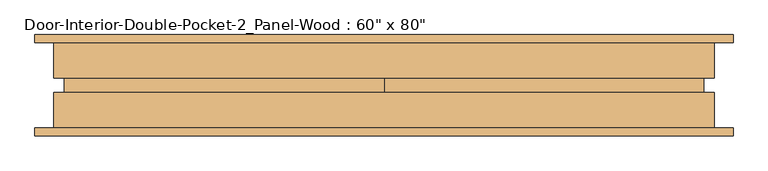
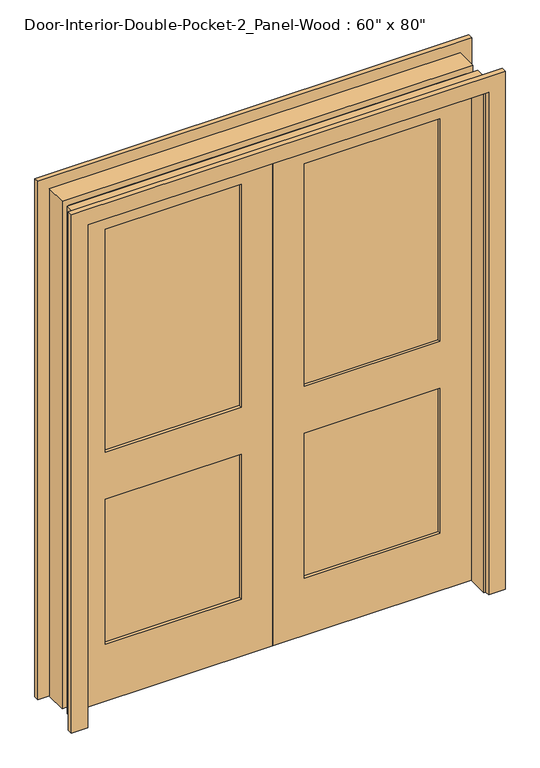
"""IFC4 building model written with IfcOpenShell, lengths in millimetres: door geometry."""

from ifc_helpers import new_model, si_unit, frame, origin, place, context, project, spatial, polyline, outline, extrude, source, transform, mapped, element, save


def door_4110a08e(model_context):
    return source(origin(), model_context, "Body", "SweptSolid", [
        extrude(outline(polyline([(0.0, 768.35), (0.0, 831.85), (2101.85, 831.85), (2101.85, -831.85), (0.0, -831.85), (0.0, -768.35), (2038.35, -768.35), (2038.35, 768.35), (0.0, 768.35)])), frame((0.0, -120.65, 0.0), z_axis=(0.0, 1.0, 0.0), x_axis=(0.0, 0.0, 1.0)), (0.0, 0.0, 1.0), 19.05),
        extrude(outline(polyline([(0.0, 768.35), (0.0, 831.85), (2101.85, 831.85), (2101.85, -831.85), (0.0, -831.85), (0.0, -768.35), (2038.35, -768.35), (2038.35, 768.35), (0.0, 768.35)])), frame((0.0, 101.6, 0.0), z_axis=(0.0, 1.0, 0.0), x_axis=(0.0, 0.0, 1.0)), (0.0, 0.0, 1.0), 19.05),
        extrude(outline(polyline([(-120.65, -5.8208333), (-641.35, -5.8208333), (-641.35, 5.8208333), (-120.65, 5.8208333), (-120.65, -5.8208333)])), frame((0.0, 0.0, 1009.65), z_axis=(0.0, 0.0, 1.0), x_axis=(1.0, 0.0, 0.0)), (0.0, 0.0, 1.0), 903.2875),
        extrude(outline(polyline([(-120.65, -5.8208333), (-641.35, -5.8208333), (-641.35, 5.8208333), (-120.65, 5.8208333), (-120.65, -5.8208333)])), frame((0.0, 0.0, 231.775), z_axis=(0.0, 0.0, 1.0), x_axis=(1.0, 0.0, 0.0)), (0.0, 0.0, 1.0), 587.375),
        extrude(outline(polyline([(2032.0, -762.0), (0.0, -762.0), (0.0, 0.0), (2032.0, 0.0), (2032.0, -762.0)]), holes=[polyline([(1912.9375, -641.35), (1912.9375, -120.65), (1009.65, -120.65), (1009.65, -641.35), (1912.9375, -641.35)]), polyline([(819.15, -641.35), (819.15, -120.65), (231.775, -120.65), (231.775, -641.35), (819.15, -641.35)])]), frame((0.0, -17.4625, 0.0), z_axis=(0.0, 1.0, 0.0), x_axis=(0.0, 0.0, 1.0)), (0.0, 0.0, 1.0), 34.925),
        extrude(outline(polyline([(0.0, 787.4), (2057.4, 787.4), (2057.4, -787.4), (0.0, -787.4), (0.0, -762.0), (2032.0, -762.0), (2032.0, 762.0), (0.0, 762.0), (0.0, 787.4)])), frame((0.0, 17.4625, 0.0), z_axis=(0.0, 1.0, 0.0), x_axis=(0.0, 0.0, 1.0)), (0.0, 0.0, 1.0), 84.1375),
        extrude(outline(polyline([(0.0, 787.4), (2057.4, 787.4), (2057.4, -787.4), (0.0, -787.4), (0.0, -762.0), (2032.0, -762.0), (2032.0, 762.0), (0.0, 762.0), (0.0, 787.4)])), frame((0.0, -101.6, 0.0), z_axis=(0.0, 1.0, 0.0), x_axis=(0.0, 0.0, 1.0)), (0.0, 0.0, 1.0), 84.1375),
        extrude(outline(polyline([(641.35, -5.8208333), (120.65, -5.8208333), (120.65, 5.8208333), (641.35, 5.8208333), (641.35, -5.8208333)])), frame((0.0, 0.0, 1009.65), z_axis=(0.0, 0.0, 1.0), x_axis=(1.0, 0.0, 0.0)), (0.0, 0.0, 1.0), 903.2875),
        extrude(outline(polyline([(641.35, -5.8208333), (120.65, -5.8208333), (120.65, 5.8208333), (641.35, 5.8208333), (641.35, -5.8208333)])), frame((0.0, 0.0, 231.775), z_axis=(0.0, 0.0, 1.0), x_axis=(1.0, 0.0, 0.0)), (0.0, 0.0, 1.0), 587.375),
        extrude(outline(polyline([(2032.0, 0.0), (0.0, 0.0), (0.0, 762.0), (2032.0, 762.0), (2032.0, 0.0)]), holes=[polyline([(1912.9375, 120.65), (1912.9375, 641.35), (1009.65, 641.35), (1009.65, 120.65), (1912.9375, 120.65)]), polyline([(819.15, 120.65), (819.15, 641.35), (231.775, 641.35), (231.775, 120.65), (819.15, 120.65)])]), frame((0.0, -17.4625, 0.0), z_axis=(0.0, 1.0, 0.0), x_axis=(0.0, 0.0, 1.0)), (0.0, 0.0, 1.0), 34.925),
    ])


if __name__ == "__main__":
    model = new_model("IFC4")
    model_context = context("Model", 3, world=origin())
    ifc_project = project(units=[si_unit("LENGTHUNIT", "METRE", prefix="MILLI")], contexts=[model_context])
    site = spatial("IfcSite", under=ifc_project)
    building = spatial("IfcBuilding", under=site)
    placement = place(None, origin())
    door_shape = door_4110a08e(model_context)
    element("IfcDoor", 1, ObjectType="Door-Interior-Double-Pocket-2_Panel-Wood : 60\" x 80\"", at=placement, inside=building, context=model_context, shape_type="MappedRepresentation", body=[
        mapped(door_shape, transform((0.0, 0.0, 0.0), x_axis=(1.0, 0.0, 0.0), y_axis=(0.0, 1.0, 0.0), z_axis=(0.0, 0.0, 1.0))),
    ])
    save(model, "model.ifc")

# Revit data of these elements
# Type "Door-Interior-Double-Pocket-2_Panel-Wood : 60\" x 80\""
#   Type Mark = "11"
#   Assembly Code = "C1020300"
#   Analytic Construction = "Wooden"
#   Top Rail = 0' - 4 11/16"
#   Thickness = 0' - 1 3/8"
#   Thermal Resistance (R) = 2.5876 (h·ft²·°F)/BTU
#   Stiles = 0' - 4 3/4"
#   Rough Width = 10' - 2"
#   Rough Height = 7' - 0 1/2"
#   Panel Width = 2' - 6"
#   Lock Rail = 0' - 7 1/2"
#   Location [instance default] = 2' - 7"
#   Height = 6' - 8"
#   Width = 5' - 0"
#   Heat Transfer Coefficient (U) = 0.3865 BTU/(h·ft²·°F)
#   Bottom Rail = 0' - 9 1/8"
#   Panel Open [instance default] = no
#   Trim Material = Cherry
#   Panel Material = Cherry
#   Frame Material = Cherry
#   Visual Light Transmittance = 0
#   Solar Heat Gain Coefficient = 0
#   Wall Closure = (empty or 0)
#   Function = (empty or 0)
# Element 1 (IfcDoor, "Door-Interior-Double-Pocket-2_Panel-Wood : 60\" x 80\"")
#   Materials on its faces: "Cherry"
# Materials
#   "Cherry": class "Wood", colour RGB 226 177 128, transparency 0, Description = "Prunus Serotina", Cost = 0
